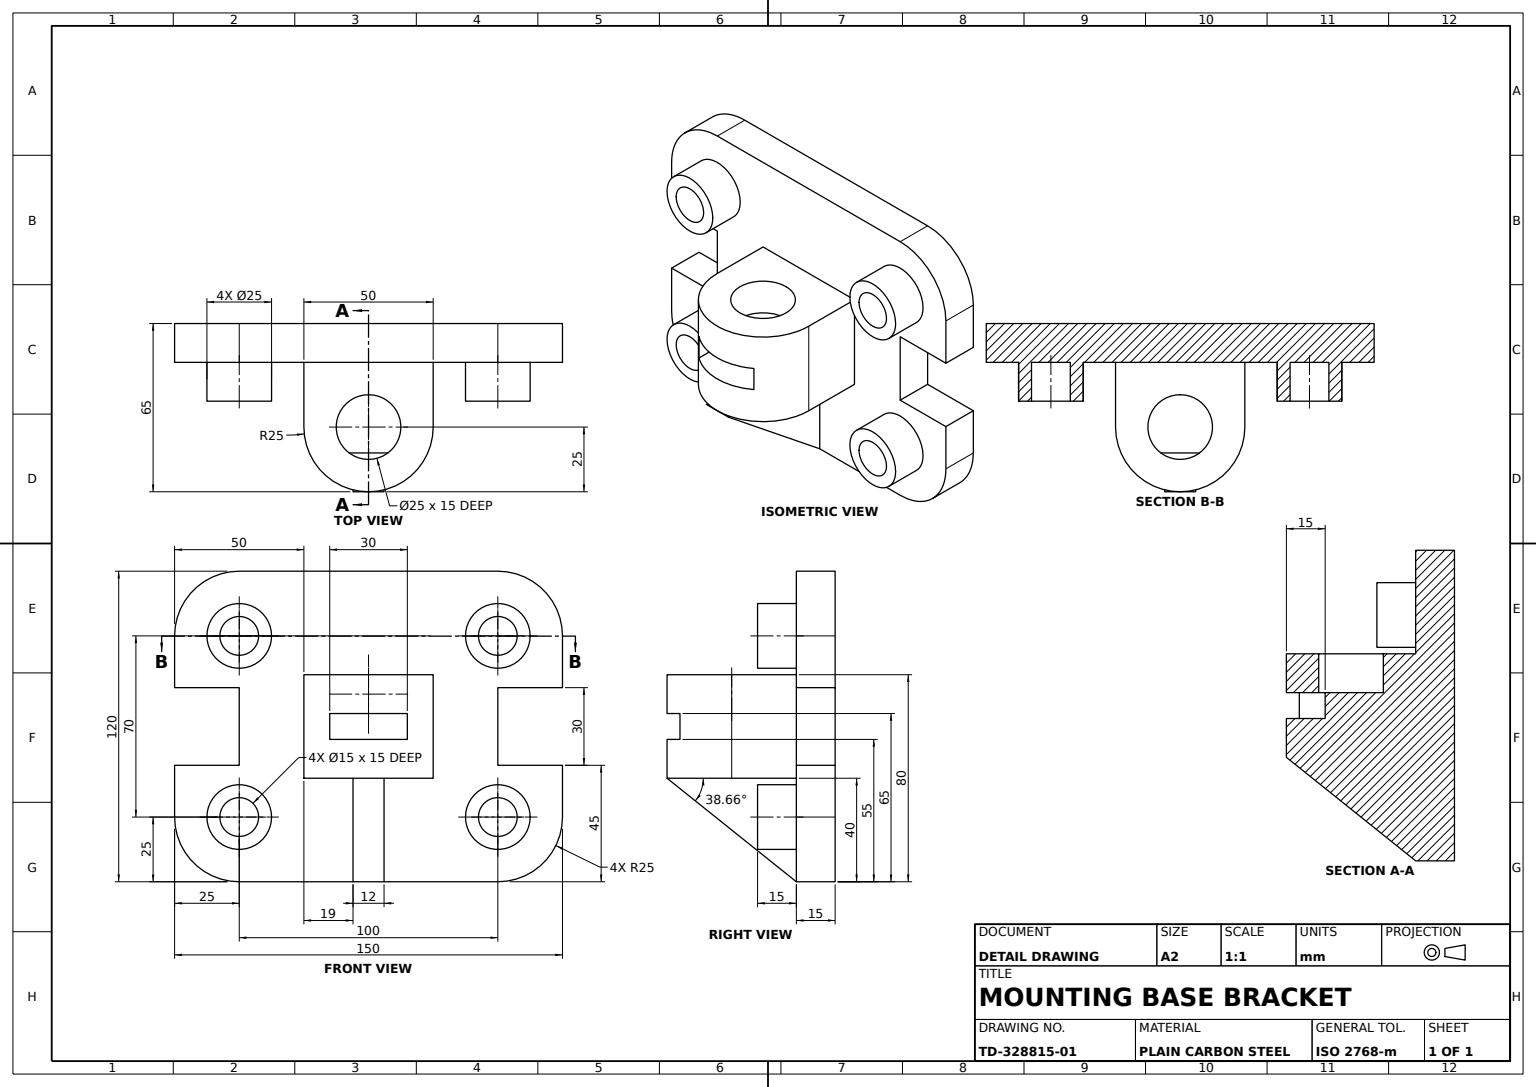
SolidWorks part; units mm, degrees
material "Plain Carbon Steel"
ref_plane "Front Plane" through (0, 0, 0) normal (0, 0, 1) x (1, 0, 0)
ref_plane "Top Plane" through (0, 0, 0) normal (0, 1, 0) x (1, 0, 0)
ref_plane "Right Plane" through (0, 0, 0) normal (1, 0, 0) x (0, 0, -1)
sketch "Base Plate Sketch" plane through (0, 0, 0) normal (0, 0, 1) x (1, 0, 0)
  line L0 (0, 0) -> (150, 0)
  line L1 (150, 0) -> (150, 120)
  line L2 (150, 120) -> (0, 120)
  line L3 (0, 120) -> (0, 0)
  dimension "D1" = 150
  dimension "D2" = 120
extrude "Base Plate 150x120x15" add sketch "Base Plate Sketch" along normal blind 15
sketch "Raised Boss Sketch" plane through (0, 0, 15) normal (0, 0, 1) x (1, 0, 0)
  line L0 (75, 60) -> (25, 60) construction
  line L1 (75, 60) -> (125, 60) construction
  line L2 (25, 60) -> (25, 95) construction
  line L3 (25, 60) -> (25, 25) construction
  line L4 (125, 60) -> (125, 95) construction
  line L5 (125, 60) -> (125, 25) construction
  line L7 (0, 0) -> (150, 0) construction
  circle A1 centre (25, 95) radius 12.5
  circle A2 centre (125, 95) radius 12.5
  circle A3 centre (125, 25) radius 12.5
  circle A4 centre (25, 25) radius 12.5
  circle A5 centre (25, 95) radius 7.5
  circle A6 centre (125, 95) radius 7.5
  circle A7 centre (25, 25) radius 7.5
  circle A8 centre (125, 25) radius 7.5
  dimension "D3" = 25
  dimension "D4" = 25
  dimension "D5" = 25
  dimension "D6" = 25
  dimension "D7" = 15
  dimension "D8" = 15
  dimension "D9" = 15
  dimension "D10" = 15
  dimension "D1" = 100
  dimension "D2" = 70
  dimension "D11" = 25
  dimension "D12" = 25
  dimension "D13" = 95
  dimension "D14" = 25
  dimension "D15" = 60
extrude "Raised Boss 15mm" add sketch "Raised Boss Sketch" along normal blind 15
ref_plane "Bearing Block Plane" through (0, 60, 0) normal (0, 1, 0) x (1, 0, 0)
sketch "Bearing Block Sketch" plane through (0, 60, 0) normal (0, 1, 0) x (1, 0, 0)
  line L0 (0, 0) -> (150, 0) construction
  line L1 (50, -40) -> (50, -15)
  line L2 (0, -15) -> (150, -15) construction
  line L3 (100, -40) -> (100, -15)
  line L4 (50, -15) -> (100, -15)
  arc A1 (50, -40) -> (100, -40) centre (75, -40) ccw
  point P5 (75, 0)
  dimension "D1" = 40
  dimension "D3" = 50
  dimension "D4" = 40
extrude "Bearing Block" add sketch "Bearing Block Sketch" along normal mid plane 40
ref_plane "Relief Cut Plane" through (0, 0, 15) normal (0, 0, 1) x (1, 0, 0)
sketch "Relief Cut Sketch" plane through (0, 0, 15) normal (0, 0, 1) x (1, 0, 0)
  line L2 (0, 120) -> (0, 0) construction
  line L4 (150, 60) -> (150, 75)
  line L5 (150, 0) -> (150, 120) construction
  line L6 (150, 60) -> (150, 45)
  line L7 (0, 75) -> (25, 75)
  line L8 (25, 75) -> (25, 45)
  line L9 (25, 45) -> (0, 45)
  line L10 (0, 75) -> (0, 45)
  line L11 (150, 75) -> (125, 75)
  line L12 (125, 75) -> (125, 45)
  line L13 (125, 45) -> (150, 45)
  dimension "D1" = 45
  dimension "D2" = 75
  dimension "D3" = 25
  dimension "D4" = 75
  dimension "D5" = 45
  dimension "D6" = 125
extrude "Relief Cut" cut sketch "Relief Cut Sketch" against normal blind 15
fillet "Plate Corner Fillets R25" radius 25 4 edges at (0, 0, 7.5) (150, 0, 7.5) (150, 120, 7.5) (0, 120, 7.5)
ref_plane "Slot Plane" through (0, 0, 65) normal (0, 0, 1) x (1, 0, 0)
sketch "Block Slot Sketch" plane through (0, 0, 65) normal (0, 0, 1) x (1, 0, 0)
  line L0 (60, 65) -> (60, 55)
  line L1 (90, 65) -> (90, 55)
  line L3 (60, 65) -> (90, 65)
  line L5 (90, 55) -> (60, 55)
  dimension "D1" = 30
  dimension "D2" = 10
  dimension "D3" = 60
  dimension "D4" = 55
extrude "Block Slot 30x10" cut sketch "Block Slot Sketch" against normal blind 15
ref_plane "Rib Mid Plane" through (75, 0, 0) normal (1, 0, 0) x (0, 0, -1)
sketch "Support Rib Sketch" plane through (75, 0, 0) normal (1, 0, 0) x (0, 0, -1)
  line L0 (-15, 0) -> (-65, 40)
  line L1 (-65, 40) -> (-15, 40)
  line L2 (-15, 40) -> (-15, 0)
extrude "Support Rib" add sketch "Support Rib Sketch" along normal mid plane 12
sketch "Bearing Bore Sketch" plane through (0, 80, 0) normal (0, 1, 0) x (1, 0, 0)
  circle A0 centre (75, -40) radius 12.5
  dimension "D1" = 25
extrude "Bearing Bore Ø25" cut sketch "Bearing Bore Sketch" against normal blind 15
